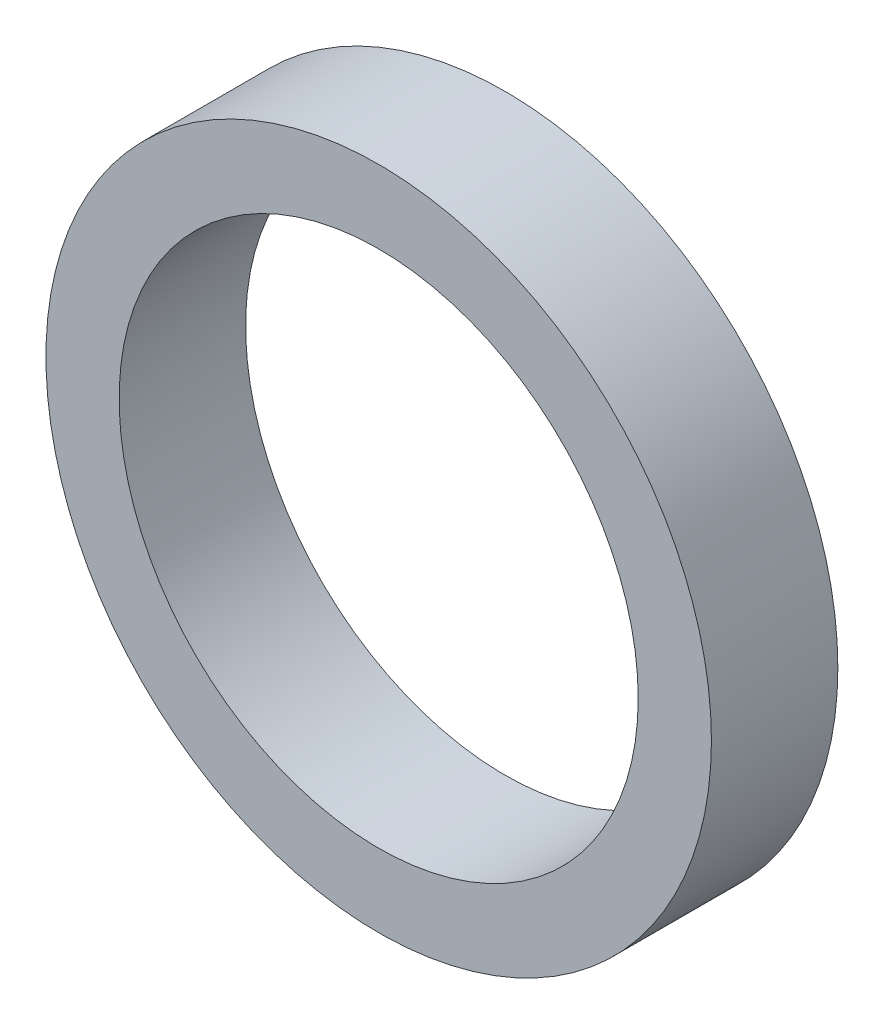
ISO-10303-21;
HEADER;
FILE_DESCRIPTION(('STEP AP214'),'2;1');
FILE_NAME('part.step','',(''),(''),'','','');
FILE_SCHEMA(('AUTOMOTIVE_DESIGN { 1 0 10303 214 1 1 1 1 }'));
ENDSEC;
DATA;
#1=APPLICATION_CONTEXT('core data for automotive mechanical design processes');
#2=APPLICATION_PROTOCOL_DEFINITION('international standard','automotive_design',2000,#1);
#3=PRODUCT_CONTEXT('',#1,'mechanical');
#4=PRODUCT('Part','Part','',(#3));
#5=PRODUCT_RELATED_PRODUCT_CATEGORY('part','',(#4));
#6=PRODUCT_DEFINITION_FORMATION('','',#4);
#7=PRODUCT_DEFINITION_CONTEXT('part definition',#1,'design');
#8=PRODUCT_DEFINITION('design','',#6,#7);
#9=PRODUCT_DEFINITION_SHAPE('','',#8);
#10=(LENGTH_UNIT() NAMED_UNIT(*) SI_UNIT(.MILLI.,.METRE.));
#11=(NAMED_UNIT(*) PLANE_ANGLE_UNIT() SI_UNIT($,.RADIAN.));
#12=(NAMED_UNIT(*) SI_UNIT($,.STERADIAN.) SOLID_ANGLE_UNIT());
#13=UNCERTAINTY_MEASURE_WITH_UNIT(LENGTH_MEASURE(1.E-05),#10,'distance_accuracy_value','');
#14=(GEOMETRIC_REPRESENTATION_CONTEXT(3) GLOBAL_UNCERTAINTY_ASSIGNED_CONTEXT((#13)) GLOBAL_UNIT_ASSIGNED_CONTEXT((#10,
#11,#12)) REPRESENTATION_CONTEXT('',''));
#15=CARTESIAN_POINT('',(0.,0.,0.));
#16=DIRECTION('',(0.,0.,1.));
#17=DIRECTION('',(1.,0.,0.));
#18=AXIS2_PLACEMENT_3D('',#15,#16,#17);
#19=CARTESIAN_POINT('',(0.,0.,2.413));
#20=DIRECTION('',(0.,0.,1.));
#21=DIRECTION('',(1.,0.,0.));
#22=AXIS2_PLACEMENT_3D('',#19,#20,#21);
#23=PLANE('',#22);
#24=CARTESIAN_POINT('',(0.,0.,2.413));
#25=DIRECTION('',(0.,0.,1.));
#26=DIRECTION('',(1.,0.,0.));
#27=AXIS2_PLACEMENT_3D('',#24,#25,#26);
#28=CIRCLE('',#27,6.35);
#29=CARTESIAN_POINT('',(6.35,0.,2.413));
#30=VERTEX_POINT('',#29);
#31=EDGE_CURVE('E10',#30,#30,#28,.T.);
#32=ORIENTED_EDGE('',*,*,#31,.T.);
#33=EDGE_LOOP('',(#32));
#34=FACE_BOUND('',#33,.T.);
#35=CARTESIAN_POINT('',(0.,0.,2.413));
#36=DIRECTION('',(0.,0.,1.));
#37=DIRECTION('',(1.,0.,0.));
#38=AXIS2_PLACEMENT_3D('',#35,#36,#37);
#39=CIRCLE('',#38,4.953);
#40=CARTESIAN_POINT('',(4.953,0.,2.413));
#41=VERTEX_POINT('',#40);
#42=EDGE_CURVE('E48',#41,#41,#39,.T.);
#43=ORIENTED_EDGE('',*,*,#42,.F.);
#44=EDGE_LOOP('',(#43));
#45=FACE_BOUND('',#44,.T.);
#46=ADVANCED_FACE('F40',(#34,#45),#23,.T.);
#47=CARTESIAN_POINT('',(0.,0.,0.));
#48=DIRECTION('',(0.,0.,1.));
#49=DIRECTION('',(1.,0.,0.));
#50=AXIS2_PLACEMENT_3D('',#47,#48,#49);
#51=PLANE('',#50);
#52=CARTESIAN_POINT('',(0.,0.,0.));
#53=DIRECTION('',(0.,0.,1.));
#54=DIRECTION('',(1.,0.,0.));
#55=AXIS2_PLACEMENT_3D('',#52,#53,#54);
#56=CIRCLE('',#55,6.35);
#57=CARTESIAN_POINT('',(6.35,0.,0.));
#58=VERTEX_POINT('',#57);
#59=EDGE_CURVE('E41',#58,#58,#56,.T.);
#60=ORIENTED_EDGE('',*,*,#59,.F.);
#61=EDGE_LOOP('',(#60));
#62=FACE_BOUND('',#61,.T.);
#63=CARTESIAN_POINT('',(0.,0.,0.));
#64=DIRECTION('',(0.,0.,1.));
#65=DIRECTION('',(1.,0.,0.));
#66=AXIS2_PLACEMENT_3D('',#63,#64,#65);
#67=CIRCLE('',#66,4.953);
#68=CARTESIAN_POINT('',(4.953,0.,0.));
#69=VERTEX_POINT('',#68);
#70=EDGE_CURVE('E49',#69,#69,#67,.T.);
#71=ORIENTED_EDGE('',*,*,#70,.T.);
#72=EDGE_LOOP('',(#71));
#73=FACE_BOUND('',#72,.T.);
#74=ADVANCED_FACE('F58',(#62,#73),#51,.F.);
#75=CARTESIAN_POINT('',(0.,0.,2.413));
#76=DIRECTION('',(0.,0.,-1.));
#77=DIRECTION('',(-1.,0.,0.));
#78=AXIS2_PLACEMENT_3D('',#75,#76,#77);
#79=CYLINDRICAL_SURFACE('',#78,6.35);
#80=ORIENTED_EDGE('',*,*,#31,.F.);
#81=EDGE_LOOP('',(#80));
#82=FACE_BOUND('',#81,.T.);
#83=ORIENTED_EDGE('',*,*,#59,.T.);
#84=EDGE_LOOP('',(#83));
#85=FACE_BOUND('',#84,.T.);
#86=ADVANCED_FACE('F39',(#82,#85),#79,.T.);
#87=CARTESIAN_POINT('',(0.,0.,2.413));
#88=DIRECTION('',(0.,0.,-1.));
#89=DIRECTION('',(-1.,0.,0.));
#90=AXIS2_PLACEMENT_3D('',#87,#88,#89);
#91=CYLINDRICAL_SURFACE('',#90,4.953);
#92=ORIENTED_EDGE('',*,*,#42,.T.);
#93=EDGE_LOOP('',(#92));
#94=FACE_BOUND('',#93,.T.);
#95=ORIENTED_EDGE('',*,*,#70,.F.);
#96=EDGE_LOOP('',(#95));
#97=FACE_BOUND('',#96,.T.);
#98=ADVANCED_FACE('F57',(#94,#97),#91,.F.);
#99=CLOSED_SHELL('',(#46,#74,#86,#98));
#100=MANIFOLD_SOLID_BREP('B2',#99);
#101=ADVANCED_BREP_SHAPE_REPRESENTATION('',(#18,#100),#14);
#102=SHAPE_DEFINITION_REPRESENTATION(#9,#101);
ENDSEC;
END-ISO-10303-21;
